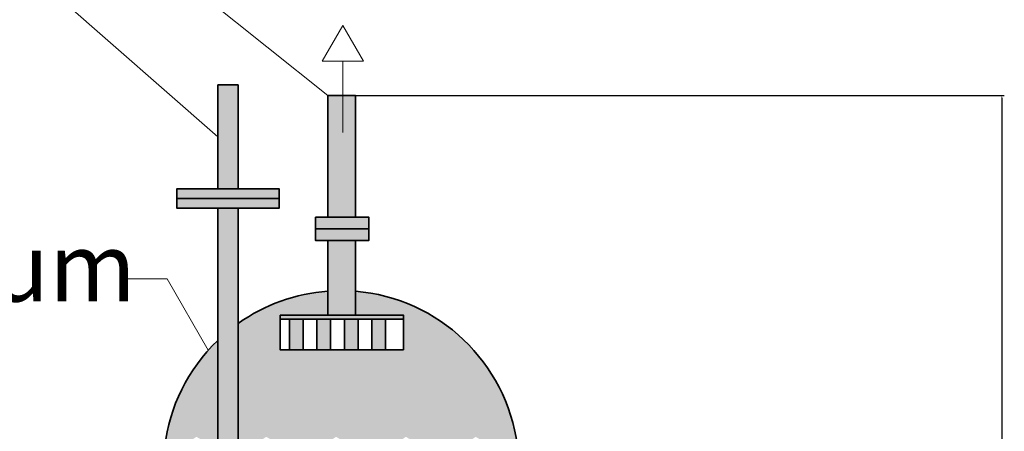
# Model space of a CAD drawing. Units: inches. Extents: x -1 to 292, y -3 to 199.
# Tile 51 of 52: x 220 to 292, y 101 to 131. Entities that reach past the tile are written whole.
import ezdxf

# ---------------------------------------------------------------- set-up
doc = ezdxf.new("R2010")
doc.units = ezdxf.units.IN
doc.header["$MEASUREMENT"] = 0
for name, color, linetype, lineweight in [('M-ANNO-LEAD', 2, 'Continuous', 18), ('M-ANNO-SYMB', 1, 'Continuous', 18), ('M-ANNO-TEXT', 3, 'Continuous', 25), ('M-DIMS', 2, 'Continuous', 18), ('M-EQPM', 7, 'Continuous', 35), ('M-PATT', 8, 'Continuous', 13)]:
    doc.layers.add(name, color=color, linetype=linetype, lineweight=lineweight)
doc.styles.get("Standard").update_dxf_attribs({"font": 'arial.ttf'})
doc.dimstyles.get("Standard").update_dxf_attribs({"dimtxt": 0.18, "dimasz": 0.18, "dimexe": 0.18, "dimexo": 0.0625, "dimgap": 0.09, "dimtad": 0, "dimtih": 1, "dimtoh": 1, "dimdec": 4, "dimzin": 0, "dimdsep": 46, "dimtxsty": 'Standard', "dimcen": 0.09, "dimadec": 0, "dimazin": 0, "dimtfac": 1, "dimtdec": 4, "dimtofl": 0, "dimtmove": 0, "dimatfit": 3, "dimfxl": 1, "dimtolj": 1, "dimtzin": 0, "dimarcsym": 0})

# ---------------------------------------------------------------- blocks, each defined once
blk = doc.blocks.new('ARROW-STEAM-OUT')
blk.add_line((113.608, 129.862), (113.608, 124.666))
blk.add_lwpolyline([(112.108, 129.862), (115.108, 129.862), (113.608, 132.46)], close=True)
blk = doc.blocks.new('*D33')
at = {"layer": 'Defpoints', "color": 0, "transparency": 16777216}
for p in [(242.955, 125.727), (292.04, 125.727), (237.933, 30.73)]:
    blk.add_point(p, dxfattribs=at)
at = {"layer": 'M-DIMS', "color": 0, "lineweight": -2, "transparency": 16777216}
for p, q in [((243.018, 125.727), (292.22, 125.727)), ((292.04, 125.547), (292.04, 78.41)), ((292.04, 30.91), (292.04, 78.046)), ((237.996, 30.73), (292.22, 30.73))]:
    blk.add_line(p, q, dxfattribs=at)
at = {"layer": 'M-DIMS', "color": 0, "transparency": 16777216}
for points in [[(292.01, 125.547), (292.07, 125.547), (292.04, 125.727)], [(292.01, 30.91), (292.07, 30.91), (292.04, 30.73)]]:
    blk.add_solid(points, dxfattribs=at)
at = {"layer": 'M-DIMS', "color": 0, "transparency": 16777216, "insert": (292.04, 78.228), "char_height": 0.18, "attachment_point": 5}
blk.add_mtext('\\A1;95', dxfattribs=at)

msp = doc.modelspace()

# ---------------------------------------------------------------- hatches: boundary and pattern name
at = {"layer": 'M-PATT'}
h = msp.add_hatch(color=256, dxfattribs=at)
h.set_gradient(color1=(0, 127, 0), color2=(0, 127, 0), tint=1, name='CYLINDER')
h.paths.add_polyline_path([(164.5186, 119.2985), (129.9293, 119.2985), (129.9293, 117.2985), (164.1897, 117.2985)])
h.paths.add_polyline_path([(181.5897, 119.2985), (164.5186, 119.2985), (164.1897, 117.2985), (179.5897, 117.2985), (179.5897, 107.8518), (181.5897, 109.1506)])
h.paths.add_polyline_path([(181.5897, 109.1506), (179.5897, 107.8518), (179.5897, 36.2698), (198.4159, 36.2698), (198.4159, 38.2698), (181.5897, 38.2698)])
h.paths.add_polyline_path([(115.4883, 126.765), (111.4883, 126.765), (111.4883, 114.6589), (115.4883, 114.6589)])
h.paths.add_polyline_path([(123.408, 119.2985), (115.4883, 119.2985), (115.4883, 117.2985), (123.408, 117.2985)])
h.paths.add_polyline_path([(115.4883, 112.6589), (111.4883, 112.6589), (111.4883, 106.9941), (115.4883, 106.9941)])
h.paths.add_polyline_path([(120.9032, 106.9941), (106.0735, 106.9941), (106.0735, 105.9941), (120.9032, 105.9941)])
h.paths.add_polyline_path([(236.4209, 117.5104), (234.9209, 117.5104), (234.9209, 97.1861), (236.4209, 97.1861)])
h.paths.add_polyline_path([(236.4209, 126.4904), (234.9209, 126.4904), (234.9209, 118.9331), (236.4209, 118.9331)])
h.paths.add_polyline_path([(244.9552, 125.7269), (242.9552, 125.7269), (242.9552, 116.8562), (244.9552, 116.8562)])
h.paths.add_polyline_path([(244.9552, 115.1721), (242.9552, 115.1721), (242.9552, 109.7385), (244.9552, 109.7385)])
h.paths.add_polyline_path([(248.4468, 109.7385), (239.4637, 109.7385), (239.4637, 109.4289), (248.4468, 109.4289)])
h = msp.add_hatch(color=256, dxfattribs=at)
h.set_gradient(color1=(209, 156, 199), color2=(0, 255, 255), tint=1, name='CYLINDER')
h.paths.add_polyline_path([(239.3906, 118.9331), (231.9512, 118.9331), (231.9512, 118.2218), (239.3906, 118.2218)])
h.paths.add_polyline_path([(239.3906, 118.2218), (231.9512, 118.2218), (231.9512, 117.5104), (234.9209, 117.5104), (239.3906, 117.5104)])
h.paths.add_polyline_path([(245.9371, 116.8562), (242.0377, 116.8562), (242.0377, 116.0141), (245.9371, 116.0141)])
h.paths.add_polyline_path([(245.9371, 116.0141), (242.0377, 116.0141), (242.0377, 115.1721), (245.9371, 115.1721)])
h = msp.add_hatch(color=256, dxfattribs=at)
h.set_gradient(color1=(209, 156, 199), color2=(0, 255, 255), tint=1, name='CYLINDER')
h.paths.add_polyline_path([(117.4883, 114.6589), (111.4883, 114.6589), (109.4883, 114.6589), (109.4883, 113.6589), (117.4883, 113.6589)])
h.paths.add_polyline_path([(117.4883, 113.6589), (109.4883, 113.6589), (109.4883, 112.6589), (115.4883, 112.6589), (117.4883, 112.6589)])
h.paths.add_polyline_path([(107.9079, 105.9941), (106.9079, 105.9941), (106.9079, 103.3981), (107.9079, 103.3981)])
h.paths.add_polyline_path([(109.9079, 105.9941), (108.9079, 105.9941), (108.9079, 103.3981), (109.9079, 103.3981)])
h.paths.add_polyline_path([(111.9079, 105.9941), (110.9079, 105.9941), (110.9079, 103.3981), (111.9079, 103.3981)])
h.paths.add_polyline_path([(113.9079, 105.9941), (112.9079, 105.9941), (112.9079, 103.3981), (113.9079, 103.3981)])
h.paths.add_polyline_path([(115.9079, 105.9941), (114.9079, 105.9941), (114.9079, 103.3981), (115.9079, 103.3981)])
h.paths.add_polyline_path([(117.9079, 105.9941), (116.9079, 105.9941), (116.9079, 103.3981), (117.9079, 103.3981)])
h.paths.add_polyline_path([(119.9079, 105.9941), (118.9079, 105.9941), (118.9079, 103.3981), (119.9079, 103.3981)])
h.paths.add_polyline_path([(241.1492, 109.4289), (240.1492, 109.4289), (240.1492, 107.2081), (241.1492, 107.2081)])
h.paths.add_polyline_path([(243.1492, 109.4289), (242.1492, 109.4289), (242.1492, 107.2081), (243.1492, 107.2081)])
h.paths.add_polyline_path([(245.1492, 109.4289), (244.1492, 109.4289), (244.1492, 107.2081), (245.1492, 107.2081)])
h.paths.add_polyline_path([(247.1492, 109.4289), (246.1492, 109.4289), (246.1492, 107.2081), (247.1492, 107.2081)])
h = msp.add_hatch(color=256, dxfattribs=at)
h.set_gradient(color1=(205, 32, 39), color2=(242, 113, 114), tint=1, name='CYLINDER')
h.paths.add_polyline_path([(243.5443, 100.87), (246.2365, 99.3157), (248.6299, 100.87), (251.3221, 99.3157), (253.7155, 100.87), (256.4077, 99.3157), (256.8092, 99.5764, 0.3682504), (244.9552, 111.4691), (244.9552, 109.7385), (248.4468, 109.7385), (248.4468, 107.2081), (239.4637, 107.2081), (239.4637, 109.7385), (242.9552, 109.7385), (242.9552, 111.4772, 0.1365835), (236.4209, 109.1305), (236.4209, 99.5466), (238.4587, 100.87), (241.1509, 99.3157)])
h.paths.add_polyline_path([(230.9797, 99.3157), (233.3731, 100.87), (234.9209, 99.9764), (234.9209, 107.8885, 0.1887049)])

# ---------------------------------------------------------------- linework, layer by layer
at = {"layer": 'M-ANNO-LEAD'}
for p, q in [((242.9552, 125.7269), (215.8975, 147.2795)), ((234.9209, 122.7118), (222.6022, 133.5105)), ((231.233, 112.3803), (227.9031, 112.3803)), ((234.237, 107.1773), (231.233, 112.3803))]:
    msp.add_line(p, q, dxfattribs=at)
at = {"layer": 'M-EQPM'}
for p, q in [((234.9209, 126.4904), (236.4209, 126.4904)), ((234.9209, 118.9331), (234.9209, 126.4904)), ((236.4209, 118.9331), (236.4209, 126.4904)), ((244.9552, 125.7269), (242.9552, 125.7269)), ((242.9552, 116.8562), (242.9552, 125.7269)), ((244.9552, 116.8562), (244.9552, 125.7269)), ((231.9512, 118.2218), (239.3906, 118.2218)), ((234.9209, 97.1861), (234.9209, 117.5104)), ((236.4209, 97.1861), (236.4209, 117.5104)), ((242.0377, 116.0141), (245.9371, 116.0141)), ((242.9552, 109.7385), (242.9552, 115.1721)), ((244.9552, 109.7385), (244.9552, 115.1721)), ((239.4637, 109.4289), (248.4468, 109.4289)), ((240.1492, 109.4289), (240.1492, 107.2081)), ((241.1492, 109.4289), (241.1492, 107.2081)), ((242.1492, 109.4289), (242.1492, 107.2081)), ((243.1492, 109.4289), (243.1492, 107.2081)), ((244.1492, 109.4289), (244.1492, 107.2081)), ((245.1492, 109.4289), (245.1492, 107.2081)), ((246.1492, 109.4289), (246.1492, 107.2081)), ((247.1492, 109.4289), (247.1492, 107.2081))]:
    msp.add_line(p, q, dxfattribs=at)
msp.add_lwpolyline([(234.9209, 117.5104), (231.9512, 117.5104), (231.9512, 118.9331), (239.3906, 118.9331), (239.3906, 117.5104), (234.9209, 117.5104)], dxfattribs=at)
for points in [[(242.0377, 116.8562), (245.9371, 116.8562), (245.9371, 115.1721), (242.0377, 115.1721)], [(239.4637, 109.7385), (248.4468, 109.7385), (248.4468, 107.2081), (239.4637, 107.2081)]]:
    msp.add_lwpolyline(points, close=True, dxfattribs=at)
for start, end in [(133.937432, 85.339055), (94.199907, 125.31004)]:
    msp.add_arc((243.9033, 98.5666), 12.9453, start, end, dxfattribs=at)

# ---------------------------------------------------------------- block references
at = {"layer": 'M-ANNO-SYMB'}
msp.add_blockref('ARROW-STEAM-OUT', (130.4342, -1.6433), dxfattribs=at)

# ---------------------------------------------------------------- texts
at = {"layer": 'M-ANNO-TEXT', "insert": (190.4016, 115.7236), "char_height": 5, "attachment_point": 1}
msp.add_mtext_dynamic_manual_height_columns('steam drum', width=47.899539, gutter_width=1, heights=[0], dxfattribs=at)

# ---------------------------------------------------------------- dimensions: what is measured, and where the dimension line sits
at = {"layer": 'M-DIMS'}
dim = msp.add_linear_dim(base=(292.0399, 125.7269), p1=(237.9333, 30.7296), p2=(242.9552, 125.7269), angle=90, dimstyle='Standard', override={"dimdec": 0, "dimlfac": 1, "dimrnd": 0, "dimzin": 0, "dimdsep": 46, "dimlunit": 2}, dxfattribs=at)
dim.commit()
dim.dimension.update_dxf_attribs({"geometry": '*D33', "text_midpoint": (292.0399, 78.2282)})

doc.saveas('drawing.dxf')
